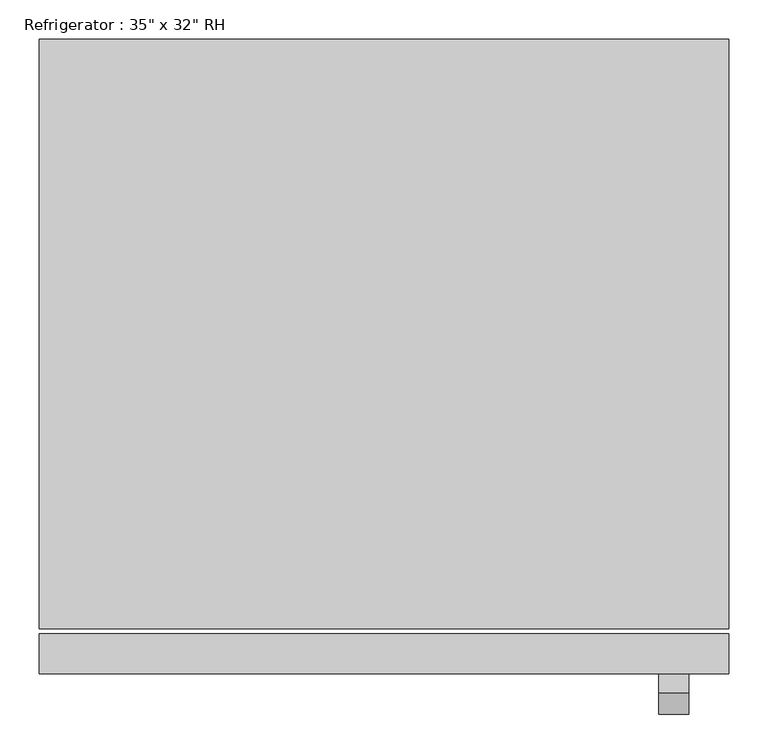
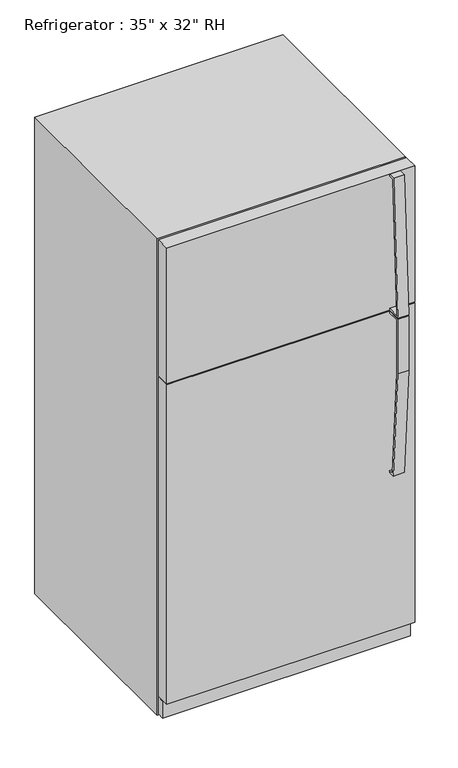
"""IFC4 building model written with IfcOpenShell, lengths in millimetres: proxy geometry."""

from ifc_helpers import new_model, si_unit, frame, origin, origin_with_axes, place, context, project, spatial, polyline, outline, extrude, source, transform, mapped, element, save


def proxy_9109806d(model_context):
    return source(origin(), model_context, "Body", "SweptSolid", [
        extrude(outline(polyline([(-417.9010285, 1262.0625), (-462.3510285, 1262.0625), (-462.3510285, 1065.4342469), (-434.8723987, 672.4715334), (-417.9010285, 672.4715334), (-417.9010285, 666.1370017), (-440.7949512, 666.1370017), (-468.7010285, 1065.2125), (-468.7010285, 1268.4125), (-417.9010285, 1268.4125), (-417.9010285, 1262.0625)])), frame((349.25, 0.0, 0.0), z_axis=(1.0, 0.0, 0.0), x_axis=(0.0, 1.0, 0.0)), (0.0, 0.0, 1.0), 38.4332978),
        extrude(outline(polyline([(-442.739413, 1778.0), (-418.6780855, 1778.0), (-418.6780855, 1771.65), (-437.5263449, 1771.65), (-463.4007207, 1277.9375), (-418.6780855, 1277.9375), (-418.6780855, 1271.5875), (-469.2793675, 1271.5875), (-442.739413, 1778.0)])), frame((349.25, 0.0, 0.0), z_axis=(1.0, 0.0, 0.0), x_axis=(0.0, 1.0, 0.0)), (0.0, 0.0, 1.0), 38.4332978),
        extrude(outline(polyline([(438.15, -367.1010285), (438.15, -392.5010285), (-438.15, -392.5010285), (-438.15, -367.1010285), (438.15, -367.1010285)])), frame((0.0, 0.0, 9.3816357), z_axis=(0.0, 0.0, 1.0), x_axis=(1.0, 0.0, 0.0)), (0.0, 0.0, 1.0), 63.5),
        extrude(outline(polyline([(438.15, -367.1010285), (438.15, -417.9010285), (-438.15, -417.9010285), (-438.15, -367.1010285), (438.15, -367.1010285)])), frame((0.0, 0.0, 76.2), z_axis=(0.0, 0.0, 1.0), x_axis=(1.0, 0.0, 0.0)), (0.0, 0.0, 1.0), 1192.2125),
        extrude(outline(polyline([(438.15, -367.1010285), (438.15, -417.9010285), (-438.15, -417.9010285), (-438.15, -367.1010285), (438.15, -367.1010285)])), frame((0.0, 0.0, 1271.5875), z_axis=(0.0, 0.0, 1.0), x_axis=(1.0, 0.0, 0.0)), (0.0, 0.0, 1.0), 506.4125),
        extrude(outline(polyline([(438.15, 388.5489715), (438.15, -360.7510285), (-438.15, -360.7510285), (-438.15, 388.5489715), (438.15, 388.5489715)])), origin_with_axes(), (0.0, 0.0, 1.0), 1778.0),
    ])


if __name__ == "__main__":
    model = new_model("IFC4")
    model_context = context("Model", 3, world=origin())
    ifc_project = project(units=[si_unit("LENGTHUNIT", "METRE", prefix="MILLI")], contexts=[model_context])
    site = spatial("IfcSite", under=ifc_project)
    building = spatial("IfcBuilding", under=site)
    placement = place(None, origin())
    proxy_shape = proxy_9109806d(model_context)
    element("IfcBuildingElementProxy", 1, Name="Refrigerator : 35\" x 32\" RH", ObjectType="Refrigerator : 35\" x 32\" RH", at=placement, inside=building, context=model_context, shape_type="MappedRepresentation", body=[
        mapped(proxy_shape, transform((0.0, 0.0, 0.0), x_axis=(1.0, 0.0, 0.0), y_axis=(0.0, 1.0, 0.0), z_axis=(0.0, 0.0, 1.0))),
    ])
    save(model, "model.ifc")

# Revit data of these elements
# Type "Refrigerator : 35\" x 32\" RH"
#   Label = "REF."
#   Assembly Code = "E1090400"
#   Depth = 2' - 7 3/4"
#   Handle = 2' - 7"
#   Height = 5' - 10"
#   Rear Clearance = 0' - 2"
#   Top Door Height = 1' - 8"
#   Width = 2' - 10 1/2"
#   Material = Steel, Paint Finish, Ivory, Glossy
#   Default Elevation = 0
# Element 1 (IfcBuildingElementProxy, "Refrigerator : 35\" x 32\" RH")
#   Materials on its faces: "Steel, Paint Finish, Ivory, Glossy", "Steel, Chrome Plated"
# Materials
#   "Steel, Paint Finish, Ivory, Glossy": class "Metal", colour RGB 247 247 239, transparency 0, Description = "Steel, paint finish, ivory, glossy", Cost = 0
#   "Steel, Chrome Plated": class "Metal", colour RGB 17 17 17, transparency 0, Description = "Chromiuim plated steel", Cost = 0
